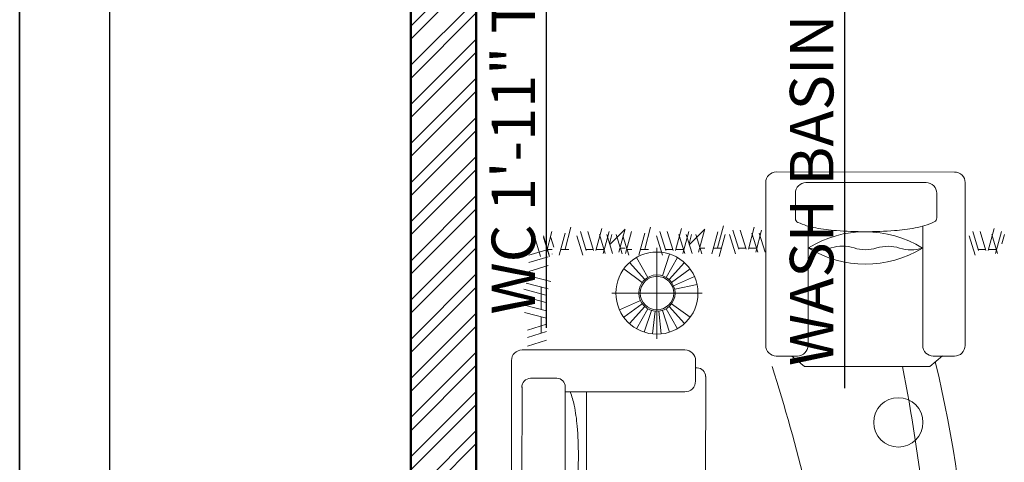
# Model space of a CAD drawing. Units: millimetres. Extents: x 20768 to 23556, y 50760 to 52704.
# Tile 17 of 36: x 21272 to 21408, y 52005 to 52066. Entities that reach past the tile are written whole.
import ezdxf

# ---------------------------------------------------------------- set-up
doc = ezdxf.new("R2010")
doc.units = ezdxf.units.MM
for name, color, linetype, lineweight in [('A-ANNO-TTLB', 7, 'Continuous', 35), ('A-FURN', 8, 'Continuous', 18), ('A-WALL', 7, 'Continuous', 50), ('A-WALL-PATT', 8, 'Continuous', 13), ('S-ANNO-DIMS', 2, 'Continuous', 18)]:
    doc.layers.add(name, color=color, linetype=linetype, lineweight=lineweight)
doc.styles.get("Standard").update_dxf_attribs({"font": 'arial.ttf'})
doc.dimstyles.new('ISO-25', dxfattribs={"dimtxt": 6, "dimasz": 2.5, "dimexe": 1.25, "dimexo": 0.625, "dimtad": 1, "dimdec": 0, "dimlunit": 3, "dimtxsty": 'Standard', "dimcen": 2.5, "dimadec": 0, "dimazin": 0, "dimtfac": 1, "dimtdec": 0, "dimtmove": 0, "dimatfit": 3, "dimfxl": 1, "dimarcsym": 0})

# ---------------------------------------------------------------- blocks, each defined once
blk = doc.blocks.new('A$C32DD204E')
for p, q in [((1063.2, 3385.6, -685.7), (1778.4, 3385.3, -685.7)), ((1020.4, 2690, -685.7), (1020.7, 3343.1, -685.7)), ((1182.2, 3343, -685.7), (1664.6, 3342.8, -685.7)), ((1820.9, 3342.8, -685.7), (1820.7, 2689.7, -685.7)), ((1139.7, 3300.5, -685.7), (1139.7, 3198.8, -685.7)), ((1707.1, 3300.3, -685.7), (1707, 3201.1, -685.7)), ((215.5, 3076.2, -685.7), (239, 3164.3, -685.7)), ((534.9, 3076.2, -685.7), (558.5, 3164.3, -685.7)), ((827.7, 3081.5, -685.7), (851.3, 3169.7, -685.7)), ((951.3, 3075.6, -685.7), (974.8, 3163.8, -685.7)), ((1190.7, 3168.5, -685.7), (1190.5, 2689.9, -685.7)), ((1650.7, 3168.4, -685.7), (1650.6, 2689.8, -685.7)), ((117, 3046.2, -685.7), (93.5, 3122.6, -685.7)), ((151.9, 3052.6, -685.7), (128.3, 3129.1, -685.7)), ((152.3, 3046.2, -685.7), (128.8, 3122.6, -685.7)), ((138.9, 3058.5, -685.7), (162.5, 3146.7, -685.7)), ((170, 3084.2, -685.7), (158.2, 3122.6, -685.7)), ((192.3, 3052.6, -685.7), (215.9, 3140.8, -685.7)), ((286.5, 3052.6, -685.7), (262.9, 3129.1, -685.7)), ((300.3, 3070.3, -685.7), (276.7, 3146.7, -685.7)), ((329.7, 3070.3, -685.7), (306.2, 3146.7, -685.7)), ((339, 3070.3, -685.7), (362.6, 3158.5, -685.7)), ((376.6, 3058.5, -685.7), (353.1, 3134.9, -685.7)), ((368.4, 3058.5, -685.7), (392, 3146.7, -685.7)), ((406, 3058.5, -685.7), (382.5, 3134.9, -685.7)), ((393.7, 3097.5, -685.7), (403.5, 3134.4, -685.7)), ((456.6, 3156.1, -685.7), (394.7, 3094.2, -685.7)), ((444.7, 3057.9, -685.7), (421.1, 3134.4, -685.7)), ((431.7, 3063.8, -685.7), (455.3, 3152, -685.7)), ((471.3, 3052.6, -685.7), (447.8, 3129.1, -685.7)), ((458.4, 3058.5, -685.7), (481.9, 3146.7, -685.7)), ((511.8, 3052.6, -685.7), (535.3, 3140.8, -685.7)), ((605.9, 3052.6, -685.7), (582.4, 3129.1, -685.7)), ((619.7, 3070.3, -685.7), (596.2, 3146.7, -685.7)), ((649.1, 3070.3, -685.7), (625.6, 3146.7, -685.7)), ((658.4, 3070.3, -685.7), (682, 3158.5, -685.7)), ((696.1, 3058.5, -685.7), (672.5, 3134.9, -685.7)), ((687.9, 3058.5, -685.7), (711.4, 3146.7, -685.7)), ((725.5, 3058.5, -685.7), (701.9, 3134.9, -685.7)), ((713.1, 3097.5, -685.7), (722.9, 3134.4, -685.7)), ((776, 3156.1, -685.7), (714.1, 3094.2, -685.7)), ((764.1, 3057.9, -685.7), (740.6, 3134.4, -685.7)), ((751.2, 3063.8, -685.7), (774.7, 3152, -685.7)), ((804.6, 3057.9, -685.7), (828.1, 3146.1, -685.7)), ((834, 3046.2, -685.7), (857.5, 3134.4, -685.7)), ((898.7, 3057.9, -685.7), (875.2, 3134.4, -685.7)), ((912.5, 3075.6, -685.7), (889, 3152, -685.7)), ((941.9, 3075.6, -685.7), (918.4, 3152, -685.7)), ((988.9, 3063.8, -685.7), (965.3, 3140.3, -685.7)), ((980.7, 3063.8, -685.7), (1004.2, 3152, -685.7)), ((1018.3, 3063.8, -685.7), (994.8, 3140.3, -685.7)), ((1861, 3052.6, -685.7), (1837.5, 3129.1, -685.7)), ((1874.9, 3070.3, -685.7), (1851.3, 3146.7, -685.7)), ((1904.3, 3070.3, -685.7), (1880.7, 3146.7, -685.7)), ((1913.6, 3070.3, -685.7), (1937.1, 3158.5, -685.7)), ((1951.2, 3058.5, -685.7), (1927.7, 3134.9, -685.7)), ((1943, 3058.5, -685.7), (1966.5, 3146.7, -685.7)), ((1968.2, 3097.5, -685.7), (1978.1, 3134.4, -685.7)), ((147, 3075.2, -685.7), (70.5, 3051.7, -685.7)), ((147, 3045.8, -685.7), (70.5, 3022.2, -685.7)), ((547.8, 2962.9, -685.7), (501.8, 3042.5, -685.7)), ((584.1, 2717, -685.7), (584.1, 3081.6, -685.7)), ((606.6, 2969.1, -685.7), (635, 3056.5, -685.7)), ((620.5, 2962.9, -685.7), (666.5, 3042.5, -685.7)), ((147, 3010.5, -685.7), (70.5, 2986.9, -685.7)), ((535.4, 2953.9, -685.7), (473.9, 3022.3, -685.7)), ((632.8, 2953.9, -685.7), (694.3, 3022.3, -685.7)), ((158.7, 2945.8, -685.7), (70.5, 2969.3, -685.7)), ((525.3, 2942.6, -685.7), (450.9, 2996.7, -685.7)), ((643, 2942.6, -685.7), (717.4, 2996.7, -685.7)), ((650.6, 2929.5, -685.7), (734.6, 2966.9, -685.7)), ((147, 2916.3, -685.7), (58.8, 2939.9, -685.7)), ((655.3, 2915, -685.7), (745.2, 2934.1, -685.7)), ((138.4, 2891.9, -685.7), (50.2, 2915.5, -685.7)), ((138.4, 2862.5, -685.7), (50.2, 2886.1, -685.7)), ((119.4, 2923.7, -685.7), (119.4, 2833.9, -685.7)), ((584.1, 2899.9, -685.7), (402.4, 2899.9, -685.7)), ((584.1, 2899.9, -685.7), (765.9, 2899.9, -685.7)), ((141.1, 2828.1, -685.7), (52.9, 2851.6, -685.7)), ((517.7, 2870.3, -685.7), (433.7, 2832.9, -685.7)), ((525.3, 2857.1, -685.7), (450.9, 2803.1, -685.7)), ((535.4, 2845.8, -685.7), (473.9, 2777.5, -685.7)), ((632.8, 2845.8, -685.7), (694.3, 2777.5, -685.7)), ((643, 2857.1, -685.7), (717.4, 2803.1, -685.7)), ((141.1, 2798.7, -685.7), (52.9, 2822.2, -685.7)), ((547.8, 2836.8, -685.7), (501.8, 2757.2, -685.7)), ((561.7, 2830.7, -685.7), (533.2, 2743.2, -685.7)), ((576.5, 2827.5, -685.7), (566.9, 2736.1, -685.7)), ((591.7, 2827.5, -685.7), (601.4, 2736.1, -685.7)), ((606.6, 2830.7, -685.7), (635, 2743.2, -685.7)), ((620.5, 2836.8, -685.7), (666.5, 2757.2, -685.7)), ((141.1, 2775.2, -685.7), (64.7, 2751.6, -685.7)), ((141.1, 2745.7, -685.7), (64.7, 2722.2, -685.7)), ((141.1, 2710.5, -685.7), (64.7, 2686.9, -685.7)), ((42.8, 2672.1, -685.7), (696.6, 2671.9, -685.7)), ((1148, 2647.4, -685.7), (1062.9, 2647.5, -685.7)), ((1125.7, 2647.4, -685.7), (1176, 2605.9, -685.7)), ((1729.9, 2647.9, -685.7), (1678.7, 2605.7, -685.7)), ((1778.1, 2647.2, -685.7), (1693.1, 2647.2, -685.7)), ((0, 755.3, -685.7), (0.2, 2629.6, -685.7)), ((739.1, 2598.6, -685.7), (739.1, 2629.3, -685.7)), ((738.8, 2602.8, -685.7), (738.8, 2546.5, -685.7)), ((739.1, 2599.7, -685.7), (745.6, 2599.7, -685.7)), ((1678.7, 2605.7, -685.7), (1176, 2605.9, -685.7)), ((76.8, 2558.3, -685.7), (182.2, 2558.3, -685.7)), ((779.4, 2042.5, -685.7), (779.6, 2565.6, -685.7)), ((42.1, 861.2, -685.7), (42.7, 2524.3, -685.7)), ((216, 1393.9, -685.7), (216.2, 2524.2, -685.7)), ((216.2, 2504.1, -685.7), (696.3, 2503.9, -685.7)), ((301, 1394, -685.7), (301.2, 2504.1, -685.7))]:
    blk.add_line(p, q)
at = {"elevation": -685.7}
for points in [[(163.7, 3074.4), (145.2, 3074.4)], [(230.7, 3074.4), (198.2, 3074.4)], [(328.4, 3074.4), (299, 3074.4)], [(372.7, 3074.4), (340.1, 3074.4)], [(371.7, 3074.4), (341.6, 3074.4)], [(456.5, 3079.7), (438, 3079.7)], [(483.2, 3074.4), (464.6, 3074.4)], [(550.1, 3074.4), (517.6, 3074.4)], [(647.8, 3074.4), (618.4, 3074.4)], [(692.1, 3074.4), (659.6, 3074.4)], [(691.2, 3074.4), (661, 3074.4)], [(776, 3079.7), (757.4, 3079.7)], [(842.9, 3079.7), (810.4, 3079.7)], [(940.6, 3079.7), (911.2, 3079.7)], [(984.9, 3079.7), (952.4, 3079.7)], [(984, 3079.7), (953.8, 3079.7)], [(1903, 3074.4), (1873.6, 3074.4)], [(1947.3, 3074.4), (1914.7, 3074.4)], [(1946.3, 3074.4), (1916.2, 3074.4)], [(119.4, 2804.5), (119.4, 2739.1)]]:
    blk.add_lwpolyline(points, dxfattribs=at)
blk.add_lwpolyline([(268.9, 2248, 0.02107), (264, 2366.2, 0.029233), (251.9, 2450.6, 0.045778), (235.8, 2504.1, 0.201615)], format="xyb", dxfattribs=at)
for centre, radius in [((584.1, 2899.9, -685.7), 164.7), ((584.1, 2899.9, -685.7), 72.8), ((584.1, 2899.9, -685.7), 67.2), ((1552.8, 2381.6, -685.7), 98.8)]:
    blk.add_circle(centre, radius)
for centre, radius, start, end in [((1063.2, 3343.1, -685.7), 42.5, 89.9772, 179.9772), ((1778.4, 3342.8, -685.7), 42.5, 359.9772, 89.9772), ((1182.2, 3300.5, -685.7), 42.5, 89.9772, 179.9772), ((1664.6, 3300.3, -685.7), 42.5, 359.9772, 89.9772), ((1690, 3201.1, -685.7), 17, 294.8183, 359.9772), ((1156.7, 3198.8, -685.7), 17, 179.9772, 246.2626), ((1280.5, 3480.4, -685.7), 324.6, 246.2626, 259.4626), ((1364.6, 3932.6, -685.7), 784.5, 259.4626, 265.581), ((1477.2, 3932.5, -685.7), 784.5, 274.3734, 280.4917), ((1560.9, 3480.3, -685.7), 324.6, 280.4917, 294.8183), ((1419.8, 2711.8, -685.7), 434.1, 58.112, 121.6703), ((1421.2, 4664.8, -685.7), 1518.9, 265.581, 269.9772), ((1421.2, 4664.8, -685.7), 1518.9, 269.9772, 274.3734), ((1329, 2937, -685.7), 151.1, 72.2902, 107.4922), ((1511.8, 2936.6, -685.7), 151.1, 72.2902, 107.4922), ((-2552.3, 2006.2, -685.7), 2911.9, 21.1287, 21.1635), ((1421.2, 3449.8, -685.7), 434.1, 238.112, 301.6703), ((1238.2, 3225.1, -685.7), 151.1, 252.2902, 287.4922), ((1420.9, 3224.8, -685.7), 151.1, 252.2902, 287.4922), ((1603.7, 3224.4, -685.7), 151.1, 252.2902, 287.4922), ((1063, 2690, -685.7), 42.5, 179.9772, 269.9772), ((1148, 2690, -685.7), 42.5, 269.9772, 359.9772), ((1693.1, 2689.7, -685.7), 42.5, 179.9772, 269.9772), ((1778.1, 2689.7, -685.7), 42.5, 269.9772, 359.9772), ((42.8, 2629.6, -685.7), 42.5, 89.9772, 179.9772), ((696.5, 2629.3, -685.7), 42.5, 359.9772, 89.9772), ((-3160.4, 1453.5, -685.7), 5000.5, 351.7639, 13.5399), ((745.5, 2565.7, -685.7), 34, 359.9772, 89.9772), ((-5717.4, 460.8, -685.7), 7095.9, 9.37507, 17.5955), ((-6034.3, 1118.6, -685.7), 7747.5, 6.78419, 11.06631), ((77.2, 2523, -685.7), 35.2, 90.762, 182.1128), ((182.2, 2524.2, -685.7), 34, 359.9772, 89.9772), ((696.3, 2546.5, -685.7), 42.5, 269.9772, 359.9772), ((-1135.1, 2248.6, -685.7), 1404, 355.1489, 359.9772)]:
    blk.add_arc(centre, radius, start, end)
blk = doc.blocks.new('*D197')
at = {"layer": 'Defpoints', "color": 0, "transparency": 16777216}
for p in [(21388.36, 52143.88), (21385.47, 52124.58), (21388.36, 52124.58)]:
    blk.add_point(p, dxfattribs=at)
at = {"layer": 'S-ANNO-DIMS', "color": 0, "lineweight": -2, "transparency": 16777216}
for p, q in [((21387.74, 52143.88), (21384.22, 52143.88)), ((21385.47, 52141.38), (21385.47, 52127.08)), ((21387.74, 52124.58), (21384.22, 52124.58)), ((21385.47, 52124.58), (21385.47, 52015.08))]:
    blk.add_line(p, q, dxfattribs=at)
at = {"layer": 'S-ANNO-DIMS', "color": 0, "transparency": 16777216}
for points in [[(21385.05, 52141.38), (21385.88, 52141.38), (21385.47, 52143.88)], [(21385.05, 52127.08), (21385.88, 52127.08), (21385.47, 52124.58)]]:
    blk.add_solid(points, dxfattribs=at)
at = {"layer": 'S-ANNO-DIMS', "color": 0, "transparency": 16777216, "insert": (21381.74, 52068.58), "char_height": 6, "attachment_point": 5, "rotation": 90}
blk.add_mtext('WASH BASIN 1\'-7 1/2" TYP.', dxfattribs=at)
blk = doc.blocks.new('*D199')
at = {"layer": 'Defpoints', "color": 0, "transparency": 16777216}
for p in [(21347.84, 52108.03), (21344.37, 52084.9), (21347.84, 52084.9)]:
    blk.add_point(p, dxfattribs=at)
at = {"layer": 'S-ANNO-DIMS', "color": 0, "lineweight": -2, "transparency": 16777216}
for p, q in [((21347.22, 52108.03), (21343.12, 52108.03)), ((21344.37, 52105.53), (21344.37, 52087.4)), ((21347.22, 52084.9), (21343.12, 52084.9)), ((21344.37, 52084.9), (21344.37, 52023.37))]:
    blk.add_line(p, q, dxfattribs=at)
at = {"layer": 'S-ANNO-DIMS', "color": 0, "transparency": 16777216}
for points in [[(21343.96, 52105.53), (21344.79, 52105.53), (21344.37, 52108.03)], [(21343.96, 52087.4), (21344.79, 52087.4), (21344.37, 52084.9)]]:
    blk.add_solid(points, dxfattribs=at)
at = {"layer": 'S-ANNO-DIMS', "color": 0, "transparency": 16777216, "insert": (21340.65, 52052.89), "char_height": 6, "attachment_point": 5, "rotation": 90}
blk.add_mtext('WC 1\'-11" TYP.', dxfattribs=at)
blk = doc.blocks.new('*D211')
at = {"layer": 'Defpoints', "color": 0, "transparency": 16777216}
for p in [(21325.74, 52522.9), (21284.24, 51829.9), (21325.74, 51829.9)]:
    blk.add_point(p, dxfattribs=at)
at = {"layer": 'S-ANNO-DIMS', "color": 0, "lineweight": -2, "transparency": 16777216}
for p, q in [((21325.12, 52522.9), (21282.99, 52522.9)), ((21284.24, 52520.4), (21284.24, 51832.4)), ((21325.12, 51829.9), (21282.99, 51829.9))]:
    blk.add_line(p, q, dxfattribs=at)
at = {"layer": 'S-ANNO-DIMS', "color": 0, "transparency": 16777216}
for points in [[(21283.82, 52520.4), (21284.66, 52520.4), (21284.24, 52522.9)], [(21283.82, 51832.4), (21284.66, 51832.4), (21284.24, 51829.9)]]:
    blk.add_solid(points, dxfattribs=at)
at = {"layer": 'S-ANNO-DIMS', "color": 0, "transparency": 16777216, "insert": (21280.55, 52176.4), "char_height": 6, "attachment_point": 5, "rotation": 90}
blk.add_mtext('57\'-9"', dxfattribs=at)
blk = doc.blocks.new('*D212')
at = {"layer": 'Defpoints', "color": 0, "transparency": 16777216}
for p in [(21334.74, 52080.4), (21284.24, 51900.4), (21334.74, 51900.4)]:
    blk.add_point(p, dxfattribs=at)
at = {"layer": 'S-ANNO-DIMS', "color": 0, "lineweight": -2, "transparency": 16777216}
for p, q in [((21334.12, 52080.4), (21282.99, 52080.4)), ((21284.24, 52077.9), (21284.24, 51902.9)), ((21334.12, 51900.4), (21282.99, 51900.4))]:
    blk.add_line(p, q, dxfattribs=at)
at = {"layer": 'S-ANNO-DIMS', "color": 0, "transparency": 16777216}
for points in [[(21283.82, 52077.9), (21284.66, 52077.9), (21284.24, 52080.4)], [(21283.82, 51902.9), (21284.66, 51902.9), (21284.24, 51900.4)]]:
    blk.add_solid(points, dxfattribs=at)
at = {"layer": 'S-ANNO-DIMS', "color": 0, "transparency": 16777216, "insert": (21280.55, 51990.4), "char_height": 6, "attachment_point": 5, "rotation": 90}
blk.add_mtext('15\'-0"', dxfattribs=at)

msp = doc.modelspace()

# ---------------------------------------------------------------- hatches: boundary and pattern name
at = {"layer": 'A-WALL-PATT'}
h = msp.add_hatch(dxfattribs=at)
h.set_pattern_fill('ANSI32', color=256, scale=0.4)
h.set_pattern_definition([(45, (-37.4434, 0), (-2.69407684, 2.69407684), []), (45, (-35.6473, 0), (-2.69407684, 2.69407684), [])])
h.paths.add_polyline_path([(21334.74, 52077.9), (21325.74, 52077.9), (21325.74, 51902.4), (21334.74, 51902.4)])

# ---------------------------------------------------------------- linework, layer by layer
at = {"layer": 'A-ANNO-TTLB'}
msp.add_line((21271.86, 52703.98), (21271.86, 51623.53), dxfattribs=at)
at = {"layer": 'A-WALL'}
for p, q in [((21325.74, 52522.9), (21325.74, 51829.9)), ((21334.74, 52513.9), (21334.74, 51829.9))]:
    msp.add_line(p, q, dxfattribs=at)

# ---------------------------------------------------------------- block references
at = {"layer": 'A-FURN', "xscale": 0.0343301531987817, "yscale": 0.0343301531987817, "zscale": 0.0343301531987817}
msp.add_blockref('A$C32DD204E', (21339.6, 51928.59, 23.54), dxfattribs=at)

# ---------------------------------------------------------------- dimensions: what is measured, and where the dimension line sits
at = {"layer": 'S-ANNO-DIMS'}
for base, p1, p2, picture, middle in [((21284.24, 51829.9), (21325.74, 52522.9), (21325.74, 51829.9), '*D211', (21280.55, 52176.4)), ((21284.24, 51900.4), (21334.74, 52080.4), (21334.74, 51900.4), '*D212', (21280.55, 51990.4))]:
    dim = msp.add_linear_dim(base=base, p1=p1, p2=p2, angle=90, dimstyle='ISO-25', override={"dimdec": 1, "dimlfac": 1, "dimrnd": 0, "dimzin": 1, "dimdsep": 46, "dimlunit": 4, "dimfrac": 2}, dxfattribs=at)
    dim.commit()
    dim.dimension.update_dxf_attribs({"geometry": picture, "text_midpoint": middle})
for base, p1, p2, text, picture, middle in [((21385.47, 52124.58), (21388.36, 52143.88), (21388.36, 52124.58), 'WASH BASIN <> TYP.', '*D197', (21381.74, 52068.58)), ((21344.37, 52084.9), (21347.84, 52108.03), (21347.84, 52084.9), 'WC <> TYP.', '*D199', (21340.65, 52052.89))]:
    dim = msp.add_linear_dim(base=base, p1=p1, p2=p2, angle=270, text=text, dimstyle='ISO-25', override={"dimdec": 1, "dimrnd": 0, "dimzin": 1, "dimlunit": 4, "dimfrac": 2}, dxfattribs=at)
    dim.commit()
    dim.dimension.update_dxf_attribs({"geometry": picture, "text_midpoint": middle})

doc.saveas('drawing.dxf')
